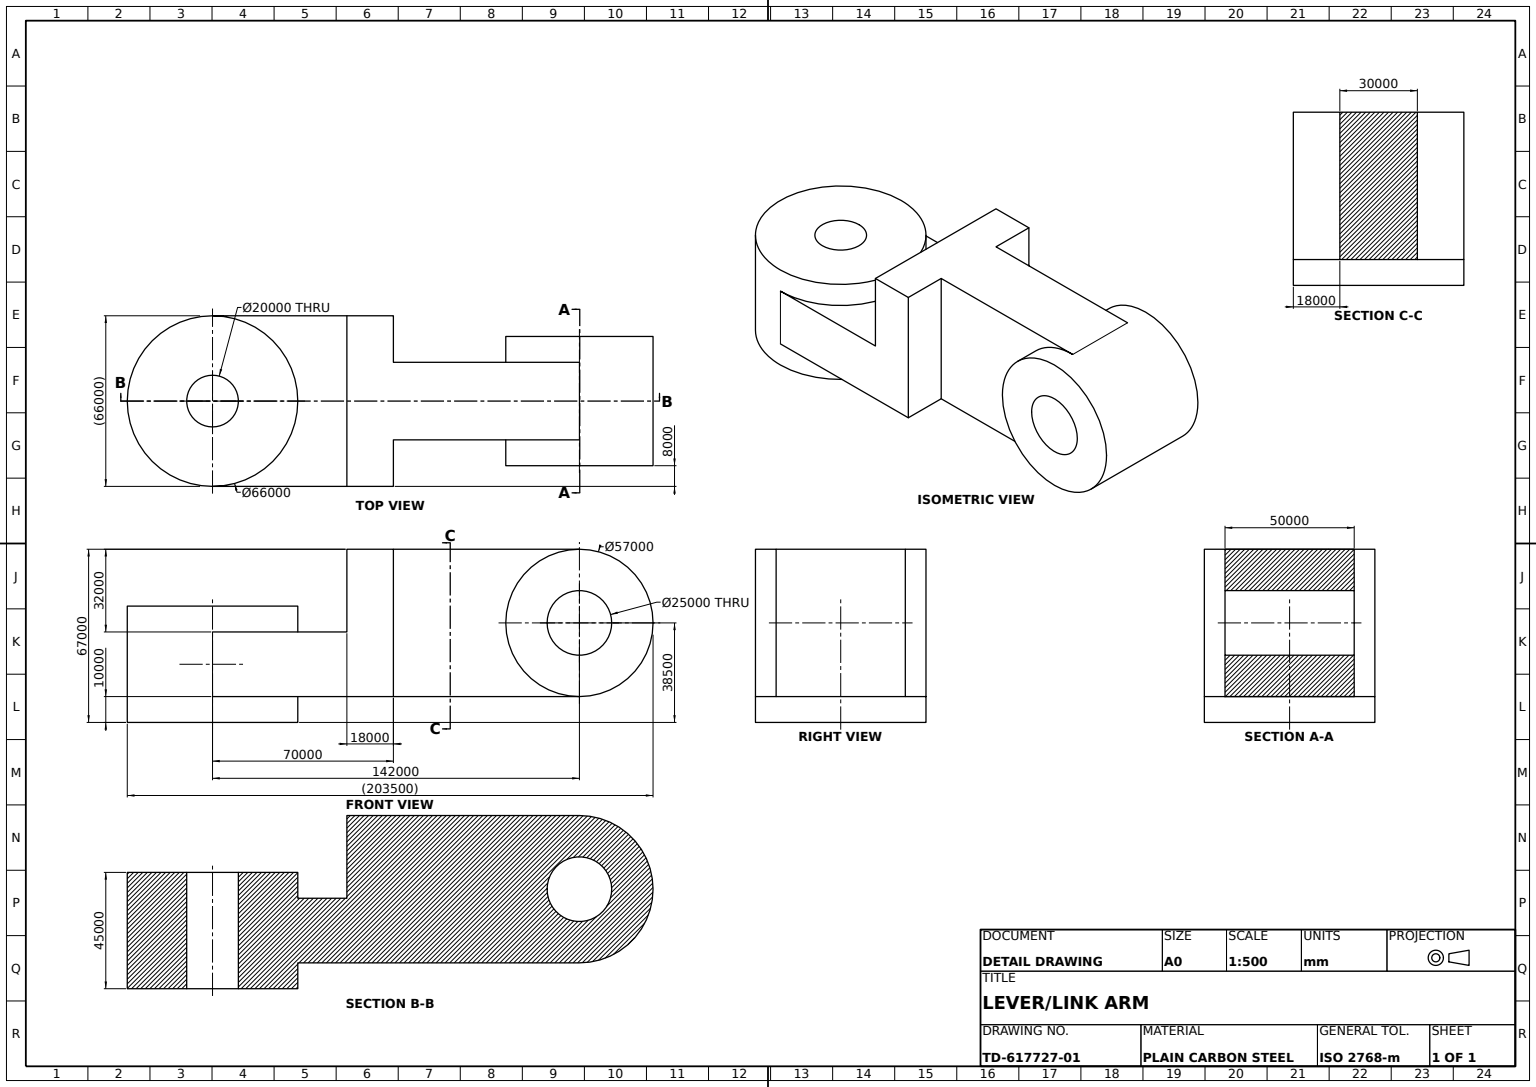
SolidWorks part; units mm, degrees
material "Plain Carbon Steel"
ref_plane "Front Plane" through (0, 0, 0) normal (0, 0, 1) x (1, 0, 0)
ref_plane "Top Plane" through (0, 0, 0) normal (0, 1, 0) x (1, 0, 0)
ref_plane "Right Plane" through (0, 0, 0) normal (1, 0, 0) x (0, 0, -1)
sketch "Vertical Eye Boss Sketch Ø66" plane through (0, 0, 0) normal (0, 1, 0) x (1, 0, 0)
  circle A0 centre (0, 0) radius 33000
  dimension "D1" = 66000
extrude "Vertical Eye Boss Ø66" add sketch "Vertical Eye Boss Sketch Ø66" along normal mid plane 45000
sketch "Vertical Eye Bore Sketch Ø20" plane through (0, 22500, 0) normal (0, 1, 0) x (1, 0, 0)
  circle A0 centre (0, 0) radius 10000
  dimension "D1" = 20000
extrude "Vertical Eye Bore Ø20" cut sketch "Vertical Eye Bore Sketch Ø20" against normal blind 45000
sketch "Arm Base Sketch" plane through (0, 0, 0) normal (0, 1, 0) x (1, 0, 0)
  line L1 (0, 33000) -> (70000, 33000)
  line L3 (0, -33000) -> (70000, -33000)
  line L4 (70000, 33000) -> (70000, -33000)
  circle A0 centre (0, 0) radius 33000 construction
  arc A1 (0, -33000) -> (0, 33000) centre (0, 0) ccw
  dimension "D1" = 70000
  dimension "D2" = 66000
  dimension "D3" = 70000
extrude "Arm Base Plate" add sketch "Arm Base Sketch" along normal mid plane 25000
sketch "Arm Web Sketch" plane through (0, 12500, 0) normal (0, 1, 0) x (1, 0, 0)
  line L0 (70000, 33000) -> (0, 33000) construction
  line L1 (70000, -33000) -> (52000, -33000)
  line L2 (70000, -33000) -> (70000, 33000)
  line L3 (70000, 33000) -> (52000, 33000)
  line L4 (52000, -33000) -> (52000, 33000)
  dimension "D1" = 18000
extrude "Arm Web" add sketch "Arm Web Sketch" along normal blind 32000
sketch "Arm Rib Profile Sketch" plane through (0, 44500, 0) normal (0, 1, 0) x (1, 0, 0)
  line L5 (70000, -33000) -> (70000, 33000) construction
  line L6 (70000, 15000) -> (142000, 15000)
  line L8 (70000, 15000) -> (70000, -15000)
  line L9 (70000, -15000) -> (142000, -15000)
  line L10 (142000, 15000) -> (142000, -15000)
  line L11 (0, 0) -> (142000, 0) construction
  dimension "D1" = 142000
  dimension "D2" = 72000
  dimension "D3" = 30000
  dimension "D4" = 15000
extrude "Arm Rib" add sketch "Arm Rib Profile Sketch" against normal blind 57000
sketch "Horizontal Eye Boss Sketch" plane through (0, 0, 0) normal (0, 0, 1) x (1, 0, 0)
  line L0 (142000, -12500) -> (142000, 44500) construction
  circle A0 centre (142000, 16000) radius 28500
extrude "Horizontal Eye Boss" add sketch "Horizontal Eye Boss Sketch" along normal mid plane 50000
sketch "Horizontal Eye Bore Sketch Ø25" plane through (0, 0, 25000) normal (0, 0, 1) x (1, 0, 0)
  circle A0 centre (142000, 16000) radius 12500
  dimension "D1" = 25000
extrude "Horizontal Eye Bore Ø25" cut sketch "Horizontal Eye Bore Sketch Ø25" against normal blind 50000
